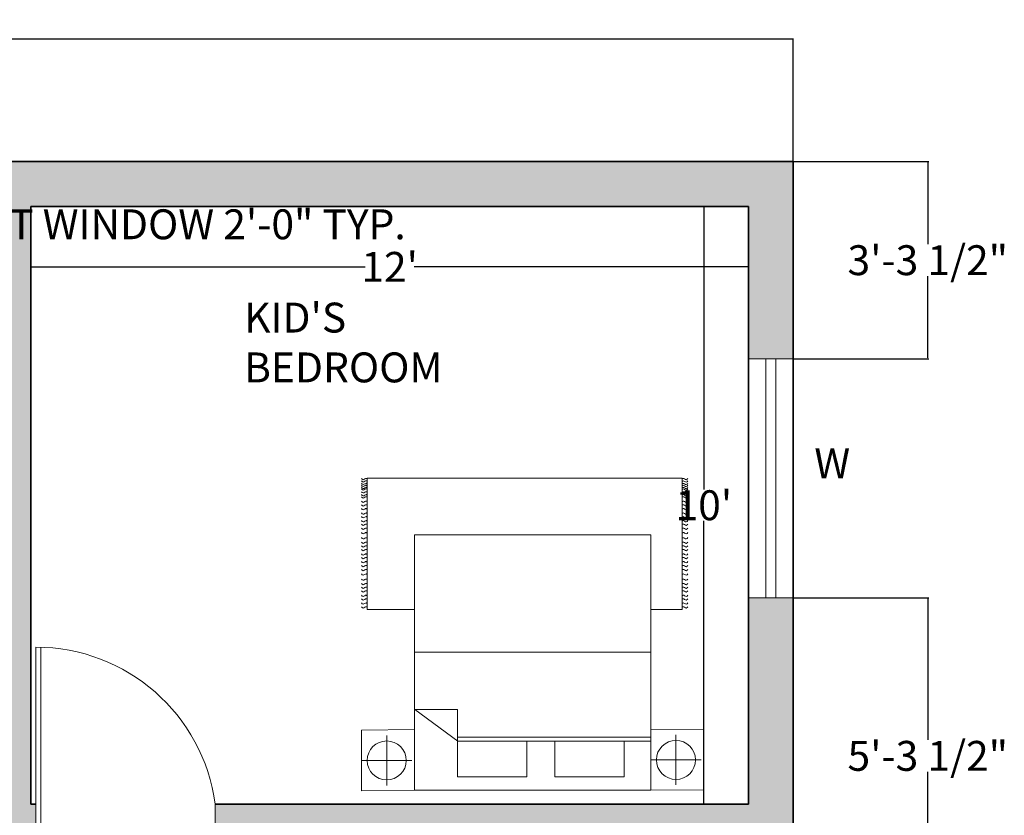
# Model space of a CAD drawing. Units: inches. Extents: x 302 to 1258, y 831 to 1373.
# Tile 6 of 13: x 569 to 767, y 1211 to 1371. Entities that reach past the tile are written whole.
import ezdxf

# ---------------------------------------------------------------- set-up
doc = ezdxf.new("R2010")
doc.units = ezdxf.units.IN
doc.header["$MEASUREMENT"] = 0
for name, color, linetype, lineweight in [('A-ANNO-DIMS', 2, 'Continuous', 18), ('A-ANNO-TEXT', 7, 'Continuous', 18), ('A-AREA-IDEN', 7, 'Continuous', 18), ('A-DOOR', 3, 'Continuous', 18), ('A-FURN', 8, 'Continuous', 18), ('A-GLAZ', 4, 'Continuous', 18), ('A-WALL', 7, 'Continuous', 35), ('A-WALL-PATT', 251, 'Continuous', 13)]:
    doc.layers.add(name, color=color, linetype=linetype, lineweight=lineweight)
doc.styles.get("Standard").update_dxf_attribs({"font": 'arial.ttf'})
doc.dimstyles.get("Standard").update_dxf_attribs({"dimtxt": 6, "dimasz": 0.18, "dimexe": 0.18, "dimexo": 0.0625, "dimgap": 0.09, "dimtad": 0, "dimtih": 1, "dimtoh": 1, "dimdec": 1, "dimzin": 0, "dimdsep": 46, "dimlunit": 3, "dimtxsty": 'Standard', "dimcen": 0.09, "dimadec": 0, "dimazin": 0, "dimtfac": 1, "dimtdec": 1, "dimtofl": 0, "dimtmove": 0, "dimatfit": 3, "dimfxl": 1, "dimtolj": 1, "dimtzin": 0, "dimarcsym": 0})

# ---------------------------------------------------------------- blocks, each defined once
blk = doc.blocks.new('*D7')
at = {"layer": 'A-ANNO-DIMS', "color": 0, "lineweight": -2, "transparency": 16777216}
for p, q in [((571.67, 1333.26), (571.67, 1320.99)), ((715.67, 1333.26), (715.67, 1320.99)), ((571.85, 1321.17), (638.77, 1321.17)), ((715.49, 1321.17), (648.57, 1321.17))]:
    blk.add_line(p, q, dxfattribs=at)
at = {"layer": 'A-ANNO-DIMS', "color": 0, "transparency": 16777216}
for points in [[(571.85, 1321.2), (571.85, 1321.14), (571.67, 1321.17)], [(715.49, 1321.2), (715.49, 1321.14), (715.67, 1321.17)]]:
    blk.add_solid(points, dxfattribs=at)
at = {"layer": 'Defpoints', "color": 0, "transparency": 16777216}
for p in [(571.67, 1333.32), (715.67, 1333.32), (715.67, 1321.17)]:
    blk.add_point(p, dxfattribs=at)
at = {"layer": 'A-ANNO-DIMS', "color": 0, "transparency": 16777216, "insert": (643.67, 1321.17), "char_height": 6, "attachment_point": 5}
blk.add_mtext("\\A1;12'", dxfattribs=at)
blk = doc.blocks.new('*D8')
at = {"layer": 'A-ANNO-DIMS', "color": 0, "lineweight": -2, "transparency": 16777216}
for p, q in [((715.61, 1333.32), (706.55, 1333.32)), ((706.73, 1333.14), (706.73, 1276.47)), ((706.73, 1213.5), (706.73, 1270.17)), ((715.61, 1213.32), (706.55, 1213.32))]:
    blk.add_line(p, q, dxfattribs=at)
at = {"layer": 'A-ANNO-DIMS', "color": 0, "transparency": 16777216}
for points in [[(706.7, 1333.14), (706.76, 1333.14), (706.73, 1333.32)], [(706.7, 1213.5), (706.76, 1213.5), (706.73, 1213.32)]]:
    blk.add_solid(points, dxfattribs=at)
at = {"layer": 'Defpoints', "color": 0, "transparency": 16777216}
for p in [(715.67, 1333.32), (706.73, 1213.32), (715.67, 1213.32)]:
    blk.add_point(p, dxfattribs=at)
at = {"layer": 'A-ANNO-DIMS', "color": 0, "transparency": 16777216, "insert": (706.73, 1273.32), "char_height": 6, "attachment_point": 5}
blk.add_mtext("\\A1;10'", dxfattribs=at)
blk = doc.blocks.new('*D31')
at = {"layer": 'A-ANNO-DIMS', "color": 0, "lineweight": -2, "transparency": 16777216}
for p, q in [((367.67, 1342.38), (367.67, 1367.04)), ((367.85, 1366.86), (532.23, 1366.86)), ((724.49, 1366.86), (560.11, 1366.86)), ((724.67, 1342.38), (724.67, 1367.04))]:
    blk.add_line(p, q, dxfattribs=at)
at = {"layer": 'A-ANNO-DIMS', "color": 0, "transparency": 16777216}
for points in [[(367.85, 1366.89), (367.85, 1366.83), (367.67, 1366.86)], [(724.49, 1366.89), (724.49, 1366.83), (724.67, 1366.86)]]:
    blk.add_solid(points, dxfattribs=at)
at = {"layer": 'Defpoints', "color": 0, "transparency": 16777216}
for p in [(724.67, 1366.86), (367.67, 1342.32), (724.67, 1342.32)]:
    blk.add_point(p, dxfattribs=at)
at = {"layer": 'A-ANNO-DIMS', "color": 0, "transparency": 16777216, "insert": (546.17, 1366.86), "char_height": 6, "attachment_point": 5}
blk.add_mtext('\\A1;29\'-9.0"', dxfattribs=at)
blk = doc.blocks.new('BED-DOUBLE-WITH-NIGHTSTANDS')
for p, q in [((1.12, 36.41), (1.12, 62.78)), ((1.12, 62.78), (64.36, 62.78)), ((64.36, 62.78), (64.36, 36.41)), ((10.66, 36.41), (1.12, 36.41)), ((64.36, 36.41), (58.06, 36.41)), ((10.66, 27.82), (58.08, 27.82)), ((19.27, 16.32), (10.71, 16.32)), ((19.32, 9.97), (10.71, 16.32)), ((19.27, 9.97), (19.27, 16.32)), ((5.06, 1.07), (5.06, 11.12)), ((19.27, 10.78), (58.08, 10.78)), ((19.32, 9.97), (58.08, 9.97)), ((63.11, 1.17), (63.11, 11.22)), ((0.03, 6.09), (10.09, 6.09)), ((58.08, 6.2), (68.14, 6.2))]:
    blk.add_line(p, q)
for points in [[(10.66, 0.1), (10.66, 51.42), (58.08, 51.42), (58.08, 0.1)], [(10.66, 12.29), (0.03, 12.19), (0.03, 0), (10.66, 0.1)], [(68.71, 12.39), (58.08, 12.29), (58.08, 0.1), (68.71, 0.2)], [(19.27, 2.8), (19.27, 9.97), (33.16, 9.97), (33.16, 2.8)], [(38.83, 2.8), (38.83, 9.97), (52.73, 9.97), (52.73, 2.8)]]:
    blk.add_lwpolyline(points, close=True)
for centre in [(5.06, 6.09), (63.11, 6.2)]:
    blk.add_circle(centre, 3.92)
for points, knots in [([(0, 62.71), (0.1, 62.59), (0.29, 62.35), (0.63, 62.59), (0.91, 62.76), (1.06, 62.66), (1.13, 62.61)], [0, 0, 0, 0, 0.400747, 0.791423, 1.067667, 1.29709, 1.29709, 1.29709, 1.29709]), ([(0, 62.24), (0.1, 62.12), (0.29, 61.88), (0.63, 62.12), (0.91, 62.29), (1.06, 62.18), (1.13, 62.13)], [0, 0, 0, 0, 0.400747, 0.791423, 1.067667, 1.29709, 1.29709, 1.29709, 1.29709]), ([(0, 61.75), (0.1, 61.63), (0.29, 61.39), (0.63, 61.63), (0.91, 61.8), (1.06, 61.7), (1.13, 61.65)], [0, 0, 0, 0, 0.400747, 0.791423, 1.067667, 1.29709, 1.29709, 1.29709, 1.29709]), ([(0, 61.35), (0.1, 61.23), (0.29, 60.99), (0.63, 61.23), (0.91, 61.41), (1.06, 61.3), (1.13, 61.25)], [0, 0, 0, 0, 0.400747, 0.791423, 1.067667, 1.29709, 1.29709, 1.29709, 1.29709]), ([(65.48, 62.71), (65.39, 62.59), (65.19, 62.35), (64.85, 62.59), (64.57, 62.76), (64.42, 62.66), (64.36, 62.61)], [0, 0, 0, 0, 0.400747, 0.791423, 1.067667, 1.29709, 1.29709, 1.29709, 1.29709]), ([(65.48, 62.21), (65.39, 62.09), (65.19, 61.85), (64.85, 62.09), (64.57, 62.26), (64.42, 62.15), (64.36, 62.11)], [0, 0, 0, 0, 0.400747, 0.791423, 1.067667, 1.29709, 1.29709, 1.29709, 1.29709]), ([(65.48, 61.72), (65.39, 61.6), (65.19, 61.36), (64.85, 61.6), (64.57, 61.78), (64.42, 61.67), (64.36, 61.62)], [0, 0, 0, 0, 0.400747, 0.791423, 1.067667, 1.29709, 1.29709, 1.29709, 1.29709]), ([(65.48, 61.33), (65.39, 61.21), (65.19, 60.97), (64.85, 61.21), (64.57, 61.38), (64.42, 61.27), (64.36, 61.22)], [0, 0, 0, 0, 0.400747, 0.791423, 1.067667, 1.29709, 1.29709, 1.29709, 1.29709]), ([(0, 60.94), (0.1, 60.81), (0.29, 60.58), (0.63, 60.81), (0.91, 60.99), (1.05, 60.89), (1.12, 60.84)], [0, 0, 0, 0, 0.400747, 0.791423, 1.067667, 1.283686, 1.283686, 1.283686, 1.283686]), ([(0, 60.63), (0.1, 60.51), (0.29, 60.27), (0.63, 60.51), (0.91, 60.68), (1.05, 60.58), (1.12, 60.53)], [0, 0, 0, 0, 0.400747, 0.791423, 1.067667, 1.283686, 1.283686, 1.283686, 1.283686]), ([(0, 60.05), (0.1, 59.93), (0.29, 59.69), (0.63, 59.93), (0.91, 60.1), (1.05, 60), (1.12, 59.96)], [0, 0, 0, 0, 0.400747, 0.791423, 1.067667, 1.283686, 1.283686, 1.283686, 1.283686]), ([(0, 59.46), (0.1, 59.34), (0.29, 59.09), (0.63, 59.34), (0.91, 59.51), (1.05, 59.41), (1.12, 59.36)], [0, 0, 0, 0, 0.402903, 0.794912, 1.071156, 1.287177, 1.287177, 1.287177, 1.287177]), ([(65.48, 60.91), (65.39, 60.79), (65.19, 60.55), (64.85, 60.79), (64.57, 60.96), (64.42, 60.85), (64.36, 60.81)], [0, 0, 0, 0, 0.400747, 0.791423, 1.067667, 1.29709, 1.29709, 1.29709, 1.29709]), ([(65.48, 60.6), (65.39, 60.48), (65.19, 60.24), (64.85, 60.48), (64.57, 60.65), (64.42, 60.54), (64.36, 60.5)], [0, 0, 0, 0, 0.400747, 0.791423, 1.067667, 1.29709, 1.29709, 1.29709, 1.29709]), ([(65.48, 60.03), (65.39, 59.9), (65.19, 59.67), (64.85, 59.9), (64.57, 60.08), (64.42, 59.97), (64.36, 59.92)], [0, 0, 0, 0, 0.400747, 0.791423, 1.067667, 1.29709, 1.29709, 1.29709, 1.29709]), ([(65.48, 59.46), (65.39, 59.33), (65.2, 59.08), (64.85, 59.34), (64.57, 59.51), (64.42, 59.4), (64.36, 59.36)], [0, 0, 0, 0, 0.407265, 0.802015, 1.07826, 1.307683, 1.307683, 1.307683, 1.307683]), ([(0, 59.03), (0.1, 58.91), (0.29, 58.67), (0.63, 58.91), (0.91, 59.08), (1.05, 58.98), (1.12, 58.93)], [0, 0, 0, 0, 0.400747, 0.791423, 1.067667, 1.283686, 1.283686, 1.283686, 1.283686]), ([(0, 58.15), (0.1, 58.03), (0.29, 57.79), (0.63, 58.03), (0.91, 58.2), (1.05, 58.1), (1.12, 58.05)], [0, 0, 0, 0, 0.400747, 0.791423, 1.067667, 1.283686, 1.283686, 1.283686, 1.283686]), ([(0, 57.42), (0.1, 57.3), (0.29, 57.06), (0.63, 57.3), (0.91, 57.47), (1.06, 57.36), (1.13, 57.32)], [0, 0, 0, 0, 0.400747, 0.791423, 1.067667, 1.29709, 1.29709, 1.29709, 1.29709]), ([(65.48, 59.03), (65.39, 58.91), (65.19, 58.67), (64.85, 58.91), (64.57, 59.08), (64.42, 58.97), (64.36, 58.93)], [0, 0, 0, 0, 0.400747, 0.791423, 1.067667, 1.29709, 1.29709, 1.29709, 1.29709]), ([(65.48, 58.15), (65.39, 58.03), (65.19, 57.79), (64.85, 58.03), (64.57, 58.2), (64.42, 58.09), (64.36, 58.04)], [0, 0, 0, 0, 0.400747, 0.791423, 1.067667, 1.29709, 1.29709, 1.29709, 1.29709]), ([(65.48, 57.42), (65.39, 57.3), (65.19, 57.06), (64.85, 57.3), (64.57, 57.47), (64.42, 57.36), (64.36, 57.32)], [0, 0, 0, 0, 0.400747, 0.791423, 1.067667, 1.29709, 1.29709, 1.29709, 1.29709]), ([(0, 56.67), (0.1, 56.55), (0.29, 56.31), (0.63, 56.55), (0.91, 56.72), (1.06, 56.61), (1.13, 56.56)], [0, 0, 0, 0, 0.400747, 0.791423, 1.067667, 1.29709, 1.29709, 1.29709, 1.29709]), ([(0, 55.78), (0.1, 55.66), (0.29, 55.42), (0.63, 55.66), (0.91, 55.84), (1.06, 55.73), (1.13, 55.68)], [0, 0, 0, 0, 0.400747, 0.791423, 1.067667, 1.29709, 1.29709, 1.29709, 1.29709]), ([(65.48, 56.67), (65.39, 56.55), (65.19, 56.31), (64.85, 56.55), (64.57, 56.72), (64.42, 56.61), (64.36, 56.56)], [0, 0, 0, 0, 0.400747, 0.791423, 1.067667, 1.29709, 1.29709, 1.29709, 1.29709]), ([(65.48, 55.78), (65.39, 55.66), (65.19, 55.42), (64.85, 55.66), (64.57, 55.84), (64.42, 55.73), (64.36, 55.68)], [0, 0, 0, 0, 0.400747, 0.791423, 1.067667, 1.29709, 1.29709, 1.29709, 1.29709]), ([(0, 55.06), (0.1, 54.94), (0.29, 54.7), (0.63, 54.94), (0.91, 55.11), (1.06, 55), (1.13, 54.95)], [0, 0, 0, 0, 0.400747, 0.791423, 1.067667, 1.29709, 1.29709, 1.29709, 1.29709]), ([(0, 54.24), (0.1, 54.12), (0.29, 53.88), (0.63, 54.12), (0.91, 54.29), (1.06, 54.19), (1.13, 54.14)], [0, 0, 0, 0, 0.400747, 0.791423, 1.067667, 1.29709, 1.29709, 1.29709, 1.29709]), ([(0, 53.55), (0.1, 53.43), (0.29, 53.19), (0.63, 53.43), (0.91, 53.6), (1.06, 53.5), (1.13, 53.45)], [0, 0, 0, 0, 0.400747, 0.791423, 1.067667, 1.29709, 1.29709, 1.29709, 1.29709]), ([(65.48, 55.06), (65.39, 54.94), (65.19, 54.7), (64.85, 54.94), (64.57, 55.11), (64.42, 55), (64.36, 54.95)], [0, 0, 0, 0, 0.400747, 0.791423, 1.067667, 1.29709, 1.29709, 1.29709, 1.29709]), ([(65.48, 54.24), (65.39, 54.12), (65.19, 53.88), (64.85, 54.12), (64.57, 54.29), (64.42, 54.19), (64.36, 54.14)], [0, 0, 0, 0, 0.400747, 0.791423, 1.067667, 1.29709, 1.29709, 1.29709, 1.29709]), ([(65.48, 53.55), (65.39, 53.43), (65.19, 53.19), (64.85, 53.43), (64.57, 53.6), (64.42, 53.5), (64.36, 53.45)], [0, 0, 0, 0, 0.400747, 0.791423, 1.067667, 1.29709, 1.29709, 1.29709, 1.29709]), ([(0, 52.73), (0.1, 52.61), (0.29, 52.37), (0.63, 52.61), (0.91, 52.79), (1.06, 52.68), (1.13, 52.63)], [0, 0, 0, 0, 0.400747, 0.791423, 1.067667, 1.29709, 1.29709, 1.29709, 1.29709]), ([(0, 51.85), (0.1, 51.73), (0.29, 51.49), (0.63, 51.73), (0.91, 51.9), (1.06, 51.8), (1.13, 51.75)], [0, 0, 0, 0, 0.400747, 0.791423, 1.067667, 1.29709, 1.29709, 1.29709, 1.29709]), ([(65.48, 52.73), (65.39, 52.61), (65.19, 52.37), (64.85, 52.61), (64.57, 52.79), (64.42, 52.68), (64.36, 52.63)], [0, 0, 0, 0, 0.400747, 0.791423, 1.067667, 1.29709, 1.29709, 1.29709, 1.29709]), ([(65.48, 51.85), (65.39, 51.73), (65.19, 51.49), (64.85, 51.73), (64.57, 51.9), (64.42, 51.8), (64.36, 51.75)], [0, 0, 0, 0, 0.400747, 0.791423, 1.067667, 1.29709, 1.29709, 1.29709, 1.29709]), ([(0, 50.82), (0.1, 50.69), (0.29, 50.46), (0.63, 50.69), (0.91, 50.87), (1.06, 50.76), (1.13, 50.71)], [0, 0, 0, 0, 0.400747, 0.791423, 1.067667, 1.29709, 1.29709, 1.29709, 1.29709]), ([(0, 49.93), (0.1, 49.81), (0.29, 49.57), (0.63, 49.81), (0.91, 49.99), (1.06, 49.88), (1.13, 49.83)], [0, 0, 0, 0, 0.400747, 0.791423, 1.067667, 1.29709, 1.29709, 1.29709, 1.29709]), ([(65.48, 50.82), (65.39, 50.69), (65.19, 50.46), (64.85, 50.69), (64.57, 50.87), (64.42, 50.76), (64.36, 50.71)], [0, 0, 0, 0, 0.400747, 0.791423, 1.067667, 1.29709, 1.29709, 1.29709, 1.29709]), ([(65.48, 49.93), (65.39, 49.81), (65.19, 49.57), (64.85, 49.81), (64.57, 49.99), (64.42, 49.88), (64.36, 49.83)], [0, 0, 0, 0, 0.400747, 0.791423, 1.067667, 1.29709, 1.29709, 1.29709, 1.29709]), ([(0, 49.21), (0.1, 49.08), (0.29, 48.84), (0.63, 49.08), (0.91, 49.26), (1.06, 49.15), (1.13, 49.1)], [0, 0, 0, 0, 0.400747, 0.791423, 1.067667, 1.29709, 1.29709, 1.29709, 1.29709]), ([(0, 48.45), (0.1, 48.33), (0.29, 48.09), (0.63, 48.33), (0.91, 48.51), (1.06, 48.4), (1.13, 48.35)], [0, 0, 0, 0, 0.400747, 0.791423, 1.067667, 1.29709, 1.29709, 1.29709, 1.29709]), ([(0, 47.57), (0.1, 47.45), (0.29, 47.21), (0.63, 47.45), (0.91, 47.62), (1.06, 47.52), (1.13, 47.47)], [0, 0, 0, 0, 0.400747, 0.791423, 1.067667, 1.29709, 1.29709, 1.29709, 1.29709]), ([(65.48, 49.21), (65.39, 49.08), (65.19, 48.84), (64.85, 49.08), (64.57, 49.26), (64.42, 49.15), (64.36, 49.1)], [0, 0, 0, 0, 0.400747, 0.791423, 1.067667, 1.29709, 1.29709, 1.29709, 1.29709]), ([(65.48, 48.45), (65.39, 48.33), (65.19, 48.09), (64.85, 48.33), (64.57, 48.51), (64.42, 48.4), (64.36, 48.35)], [0, 0, 0, 0, 0.400747, 0.791423, 1.067667, 1.29709, 1.29709, 1.29709, 1.29709]), ([(65.48, 47.57), (65.39, 47.45), (65.19, 47.21), (64.85, 47.45), (64.57, 47.62), (64.42, 47.52), (64.36, 47.47)], [0, 0, 0, 0, 0.400747, 0.791423, 1.067667, 1.29709, 1.29709, 1.29709, 1.29709]), ([(0, 46.84), (0.1, 46.72), (0.29, 46.48), (0.63, 46.72), (0.91, 46.89), (1.06, 46.79), (1.13, 46.74)], [0, 0, 0, 0, 0.400747, 0.791423, 1.067667, 1.29709, 1.29709, 1.29709, 1.29709]), ([(0, 46.03), (0.1, 45.91), (0.29, 45.67), (0.63, 45.91), (0.91, 46.08), (1.06, 45.97), (1.13, 45.92)], [0, 0, 0, 0, 0.400747, 0.791423, 1.067667, 1.29709, 1.29709, 1.29709, 1.29709]), ([(65.48, 46.84), (65.39, 46.72), (65.19, 46.48), (64.85, 46.72), (64.57, 46.89), (64.42, 46.79), (64.36, 46.74)], [0, 0, 0, 0, 0.400747, 0.791423, 1.067667, 1.29709, 1.29709, 1.29709, 1.29709]), ([(65.48, 46.03), (65.39, 45.91), (65.19, 45.67), (64.85, 45.91), (64.57, 46.08), (64.42, 45.97), (64.36, 45.92)], [0, 0, 0, 0, 0.400747, 0.791423, 1.067667, 1.29709, 1.29709, 1.29709, 1.29709]), ([(0, 45.25), (0.1, 45.13), (0.29, 44.89), (0.63, 45.13), (0.91, 45.3), (1.06, 45.2), (1.13, 45.15)], [0, 0, 0, 0, 0.400747, 0.791423, 1.067667, 1.29709, 1.29709, 1.29709, 1.29709]), ([(0, 44.43), (0.1, 44.31), (0.29, 44.07), (0.63, 44.31), (0.91, 44.49), (1.06, 44.38), (1.13, 44.33)], [0, 0, 0, 0, 0.400747, 0.791423, 1.067667, 1.29709, 1.29709, 1.29709, 1.29709]), ([(0, 43.55), (0.1, 43.43), (0.29, 43.19), (0.63, 43.43), (0.91, 43.6), (1.06, 43.5), (1.13, 43.45)], [0, 0, 0, 0, 0.400747, 0.791423, 1.067667, 1.29709, 1.29709, 1.29709, 1.29709]), ([(65.48, 45.25), (65.39, 45.13), (65.19, 44.89), (64.85, 45.13), (64.57, 45.3), (64.42, 45.2), (64.36, 45.15)], [0, 0, 0, 0, 0.400747, 0.791423, 1.067667, 1.29709, 1.29709, 1.29709, 1.29709]), ([(65.48, 44.43), (65.39, 44.31), (65.19, 44.07), (64.85, 44.31), (64.57, 44.49), (64.42, 44.38), (64.36, 44.33)], [0, 0, 0, 0, 0.400747, 0.791423, 1.067667, 1.29709, 1.29709, 1.29709, 1.29709]), ([(65.48, 43.55), (65.39, 43.43), (65.19, 43.19), (64.85, 43.43), (64.57, 43.6), (64.42, 43.5), (64.36, 43.45)], [0, 0, 0, 0, 0.400747, 0.791423, 1.067667, 1.29709, 1.29709, 1.29709, 1.29709]), ([(0, 42.52), (0.1, 42.39), (0.29, 42.15), (0.63, 42.39), (0.91, 42.57), (1.06, 42.46), (1.13, 42.41)], [0, 0, 0, 0, 0.400747, 0.791423, 1.067667, 1.29709, 1.29709, 1.29709, 1.29709]), ([(0, 41.63), (0.1, 41.51), (0.29, 41.27), (0.63, 41.51), (0.91, 41.68), (1.06, 41.58), (1.13, 41.53)], [0, 0, 0, 0, 0.400747, 0.791423, 1.067667, 1.29709, 1.29709, 1.29709, 1.29709]), ([(65.48, 42.52), (65.39, 42.39), (65.19, 42.15), (64.85, 42.39), (64.57, 42.57), (64.42, 42.46), (64.36, 42.41)], [0, 0, 0, 0, 0.400747, 0.791423, 1.067667, 1.29709, 1.29709, 1.29709, 1.29709]), ([(65.48, 41.63), (65.39, 41.51), (65.19, 41.27), (64.85, 41.51), (64.57, 41.68), (64.42, 41.58), (64.36, 41.53)], [0, 0, 0, 0, 0.400747, 0.791423, 1.067667, 1.29709, 1.29709, 1.29709, 1.29709]), ([(0, 40.9), (0.1, 40.78), (0.29, 40.54), (0.63, 40.78), (0.91, 40.96), (1.06, 40.85), (1.13, 40.8)], [0, 0, 0, 0, 0.400747, 0.791423, 1.067667, 1.29709, 1.29709, 1.29709, 1.29709]), ([(0, 40.15), (0.1, 40.03), (0.29, 39.79), (0.63, 40.03), (0.91, 40.2), (1.06, 40.1), (1.13, 40.05)], [0, 0, 0, 0, 0.400747, 0.791423, 1.067667, 1.29709, 1.29709, 1.29709, 1.29709]), ([(65.48, 40.9), (65.39, 40.78), (65.19, 40.54), (64.85, 40.78), (64.57, 40.96), (64.42, 40.85), (64.36, 40.8)], [0, 0, 0, 0, 0.400747, 0.791423, 1.067667, 1.29709, 1.29709, 1.29709, 1.29709]), ([(65.48, 40.15), (65.39, 40.03), (65.19, 39.79), (64.85, 40.03), (64.57, 40.2), (64.42, 40.1), (64.36, 40.05)], [0, 0, 0, 0, 0.400747, 0.791423, 1.067667, 1.29709, 1.29709, 1.29709, 1.29709]), ([(0, 39.27), (0.1, 39.15), (0.29, 38.91), (0.63, 39.15), (0.91, 39.32), (1.06, 39.22), (1.13, 39.17)], [0, 0, 0, 0, 0.400747, 0.791423, 1.067667, 1.29709, 1.29709, 1.29709, 1.29709]), ([(0, 38.54), (0.1, 38.42), (0.29, 38.18), (0.63, 38.42), (0.91, 38.59), (1.06, 38.49), (1.13, 38.44)], [0, 0, 0, 0, 0.400747, 0.791423, 1.067667, 1.29709, 1.29709, 1.29709, 1.29709]), ([(0, 37.73), (0.1, 37.61), (0.29, 37.37), (0.63, 37.61), (0.91, 37.78), (1.06, 37.67), (1.13, 37.62)], [0, 0, 0, 0, 0.400747, 0.791423, 1.067667, 1.29709, 1.29709, 1.29709, 1.29709]), ([(65.48, 39.27), (65.39, 39.15), (65.19, 38.91), (64.85, 39.15), (64.57, 39.32), (64.42, 39.22), (64.36, 39.17)], [0, 0, 0, 0, 0.400747, 0.791423, 1.067667, 1.29709, 1.29709, 1.29709, 1.29709]), ([(65.48, 38.54), (65.39, 38.42), (65.19, 38.18), (64.85, 38.42), (64.57, 38.59), (64.42, 38.49), (64.36, 38.44)], [0, 0, 0, 0, 0.400747, 0.791423, 1.067667, 1.29709, 1.29709, 1.29709, 1.29709]), ([(65.48, 37.73), (65.39, 37.61), (65.19, 37.37), (64.85, 37.61), (64.57, 37.78), (64.42, 37.67), (64.36, 37.62)], [0, 0, 0, 0, 0.400747, 0.791423, 1.067667, 1.29709, 1.29709, 1.29709, 1.29709]), ([(0, 36.95), (0.1, 36.83), (0.29, 36.59), (0.63, 36.83), (0.91, 37), (1.06, 36.89), (1.13, 36.85)], [0, 0, 0, 0, 0.400747, 0.791423, 1.067667, 1.29709, 1.29709, 1.29709, 1.29709]), ([(65.48, 36.95), (65.39, 36.83), (65.19, 36.59), (64.85, 36.83), (64.57, 37), (64.42, 36.89), (64.36, 36.85)], [0, 0, 0, 0, 0.400747, 0.791423, 1.067667, 1.29709, 1.29709, 1.29709, 1.29709])]:
    blk.add_open_spline(points, degree=3, knots=knots)
blk = doc.blocks.new('WINDOW-48IN')
for p, q in [((0, 0), (0, 9)), ((0, 9), (48, 9)), ((48, 9), (48, 0)), ((0, 5.5), (48, 5.5)), ((48, 3.5), (0, 3.5)), ((48, 0), (0, 0))]:
    blk.add_line(p, q)
blk = doc.blocks.new('DOOR-36IN-BEDROOM')
for p, q in [((35, 36), (35, 0)), ((36, 0), (36, 36)), ((36, 36), (36, 0)), ((0, 0), (0, 4.5)), ((36, 0), (0, 0)), ((37, 0), (36, 0))]:
    blk.add_line(p, q)
blk.add_arc((36, -0.32), 36.32, 90, 172.3719)
blk = doc.blocks.new('*D53')
at = {"layer": 'A-ANNO-DIMS', "color": 0, "lineweight": -2, "transparency": 16777216}
for p, q in [((524.78, 1333.26), (524.78, 1329.54)), ((548.78, 1333.26), (548.78, 1329.54)), ((524.96, 1329.72), (548.6, 1329.72)), ((548.78, 1329.72), (548.96, 1329.72))]:
    blk.add_line(p, q, dxfattribs=at)
at = {"layer": 'A-ANNO-DIMS', "color": 0, "transparency": 16777216}
for points in [[(524.96, 1329.75), (524.96, 1329.69), (524.78, 1329.72)], [(548.6, 1329.75), (548.6, 1329.69), (548.78, 1329.72)]]:
    blk.add_solid(points, dxfattribs=at)
at = {"layer": 'Defpoints', "color": 0, "transparency": 16777216}
for p in [(524.78, 1333.32), (548.78, 1333.32), (548.78, 1329.72)]:
    blk.add_point(p, dxfattribs=at)
at = {"layer": 'A-ANNO-DIMS', "color": 0, "transparency": 16777216, "insert": (599.38, 1329.72), "char_height": 6, "attachment_point": 5}
blk.add_mtext('\\A1;VENT WINDOW 2\'-0" TYP.', dxfattribs=at)
blk = doc.blocks.new('*D55')
at = {"layer": 'A-ANNO-DIMS', "color": 0, "lineweight": -2, "transparency": 16777216}
for p, q in [((459.67, 1208.76), (459.67, 1203.09)), ((496.67, 1208.76), (496.67, 1203.09)), ((459.85, 1203.27), (496.49, 1203.27)), ((496.67, 1203.27), (496.85, 1203.27))]:
    blk.add_line(p, q, dxfattribs=at)
at = {"layer": 'A-ANNO-DIMS', "color": 0, "transparency": 16777216}
for points in [[(459.85, 1203.3), (459.85, 1203.24), (459.67, 1203.27)], [(496.49, 1203.3), (496.49, 1203.24), (496.67, 1203.27)]]:
    blk.add_solid(points, dxfattribs=at)
at = {"layer": 'Defpoints', "color": 0, "transparency": 16777216}
for p in [(459.67, 1208.82), (496.67, 1208.82), (496.67, 1203.27)]:
    blk.add_point(p, dxfattribs=at)
at = {"layer": 'A-ANNO-DIMS', "color": 0, "transparency": 16777216, "insert": (551.65, 1203.27), "char_height": 6, "attachment_point": 5}
blk.add_mtext('\\A1;BEDROOM DOOR 3\'-1" TYP.', dxfattribs=at)
blk = doc.blocks.new('*D75')
at = {"layer": 'A-ANNO-DIMS', "color": 0, "lineweight": -2, "transparency": 16777216}
for p, q in [((724.73, 1342.32), (751.85, 1342.32)), ((751.67, 1342.14), (751.67, 1325.71)), ((751.67, 1302.89), (751.67, 1319.32)), ((724.73, 1302.71), (751.85, 1302.71))]:
    blk.add_line(p, q, dxfattribs=at)
at = {"layer": 'A-ANNO-DIMS', "color": 0, "transparency": 16777216}
for points in [[(751.64, 1342.14), (751.7, 1342.14), (751.67, 1342.32)], [(751.64, 1302.89), (751.7, 1302.89), (751.67, 1302.71)]]:
    blk.add_solid(points, dxfattribs=at)
at = {"layer": 'Defpoints', "color": 0, "transparency": 16777216}
for p in [(724.67, 1342.32), (724.67, 1302.71), (751.67, 1302.71)]:
    blk.add_point(p, dxfattribs=at)
at = {"layer": 'A-ANNO-DIMS', "color": 0, "transparency": 16777216, "insert": (751.67, 1322.51), "char_height": 6, "attachment_point": 5}
blk.add_mtext('\\A1;3\'-3 1/2"', dxfattribs=at)
blk = doc.blocks.new('*D76')
at = {"layer": 'A-ANNO-DIMS', "color": 0, "lineweight": -2, "transparency": 16777216}
for p, q in [((724.73, 1254.71), (751.85, 1254.71)), ((751.67, 1254.53), (751.67, 1226.2)), ((751.67, 1191.48), (751.67, 1219.81)), ((724.73, 1191.3), (751.85, 1191.3))]:
    blk.add_line(p, q, dxfattribs=at)
at = {"layer": 'A-ANNO-DIMS', "color": 0, "transparency": 16777216}
for points in [[(751.64, 1254.53), (751.7, 1254.53), (751.67, 1254.71)], [(751.64, 1191.48), (751.7, 1191.48), (751.67, 1191.3)]]:
    blk.add_solid(points, dxfattribs=at)
at = {"layer": 'Defpoints', "color": 0, "transparency": 16777216}
for p in [(724.67, 1254.71), (724.67, 1191.3), (751.67, 1191.3)]:
    blk.add_point(p, dxfattribs=at)
at = {"layer": 'A-ANNO-DIMS', "color": 0, "transparency": 16777216, "insert": (751.67, 1223), "char_height": 6, "attachment_point": 5}
blk.add_mtext('\\A1;5\'-3 1/2"', dxfattribs=at)

msp = doc.modelspace()

# ---------------------------------------------------------------- hatches: boundary and pattern name
at = {"layer": 'A-WALL-PATT'}
h = msp.add_hatch(color=256, dxfattribs=at)
h.dxf.hatch_style = 1
h.paths.add_polyline_path([(524.78, 1342.32), (455.57, 1342.32), (455.57, 1333.32), (496.67, 1333.32), (496.67, 1330.32), (501.17, 1330.32), (501.17, 1333.32), (524.78, 1333.32)])
h.paths.add_polyline_path([(724.67, 1342.32), (548.78, 1342.32), (548.78, 1333.32), (567.17, 1333.32), (567.17, 1213.32), (501.17, 1213.32), (501.17, 1306.32), (496.67, 1306.32), (496.67, 1213.32), (495.67, 1213.32), (495.67, 1208.82), (496.67, 1208.82), (572.67, 1208.82), (572.67, 1213.32), (571.67, 1213.32), (571.67, 1333.32), (715.67, 1333.32), (715.67, 1302.71), (724.67, 1302.71)])
h.paths.add_polyline_path([(376.67, 1333.32), (407.57, 1333.32), (407.57, 1342.32), (367.67, 1342.32), (367.67, 1300.76), (376.67, 1300.76)])
h.paths.add_polyline_path([(459.67, 1213.32), (376.67, 1213.32), (376.67, 1252.76), (367.67, 1252.76), (367.67, 1164.55), (376.67, 1164.55), (376.67, 1208.82), (454.67, 1208.82), (454.67, 1082.82), (459.17, 1082.82), (459.17, 1208.82), (459.67, 1208.82)])
h.paths.add_polyline_path([(376.67, 1116.55), (367.67, 1116.55), (367.67, 1024.44), (376.67, 1024.44)])
h.paths.add_polyline_path([(724.67, 1254.71), (715.67, 1254.71), (715.67, 1213.32), (608.67, 1213.32), (608.67, 1208.82), (615.17, 1208.82), (615.17, 1205.82), (619.67, 1205.82), (619.67, 1208.82), (715.67, 1208.82), (715.67, 1191.3), (724.67, 1191.3)])
h.paths.add_polyline_path([(724.67, 1167.3), (715.67, 1167.3), (715.67, 1136.82), (619.67, 1136.82), (619.67, 1181.82), (615.17, 1181.82), (615.17, 1136.82), (591.17, 1136.82), (591.17, 1129.32), (595.67, 1129.32), (595.67, 1132.32), (715.67, 1132.32), (715.67, 1097.42), (724.67, 1097.42)])
h.paths.add_polyline_path([(724.67, 1049.42), (715.67, 1049.42), (715.67, 1012.32), (595.67, 1012.32), (595.67, 1093.32), (591.17, 1093.32), (591.17, 1007.82), (715.67, 1007.82), (715.67, 875.82), (709.67, 875.82), (709.67, 866.82), (715.67, 866.82), (724.67, 866.82)])
h.paths.add_polyline_path([(673.67, 875.82), (623.88, 875.82), (623.88, 866.82), (673.67, 866.82)], flags=17)
h.paths.add_polyline_path([(575.88, 875.82), (477.17, 875.82), (477.17, 971.82), (472.67, 971.82), (472.67, 875.82), (376.67, 875.82), (376.67, 896.2), (367.67, 896.2), (367.67, 866.82), (575.88, 866.82)])
h.paths.add_polyline_path([(376.67, 976.44), (367.67, 976.44), (367.67, 944.2), (376.67, 944.2)])

# ---------------------------------------------------------------- linework, layer by layer
at = {"layer": 'A-WALL'}
for p, q in [((367.67, 1342.32), (724.67, 1342.32)), ((724.67, 1342.32), (724.67, 866.82)), ((571.67, 1333.32), (571.67, 1213.32)), ((571.67, 1333.32), (715.67, 1333.32)), ((715.67, 1333.32), (715.67, 1213.32)), ((571.67, 1213.32), (572.67, 1213.32)), ((608.67, 1213.32), (715.67, 1213.32))]:
    msp.add_line(p, q, dxfattribs=at)

# ---------------------------------------------------------------- block references
at = {"layer": 'A-DOOR', "extrusion": (0, 0, -1), "zscale": -1}
msp.add_blockref('DOOR-36IN-BEDROOM', (-608.67, 1208.82), dxfattribs=at)
at = {"layer": 'A-FURN'}
msp.add_blockref('BED-DOUBLE-WITH-NIGHTSTANDS', (638.02, 1215.99), dxfattribs=at)
at = {"layer": 'A-GLAZ', "rotation": 269.9999999999996}
msp.add_blockref('WINDOW-48IN', (715.67, 1302.71), dxfattribs=at)

# ---------------------------------------------------------------- texts
at = {"layer": 'A-ANNO-TEXT', "insert": (728.9, 1284.74), "char_height": 6, "attachment_point": 1}
msp.add_mtext_dynamic_manual_height_columns('W', width=16.4894, gutter_width=30, heights=[0], dxfattribs=at)
at = {"layer": 'A-AREA-IDEN', "insert": (614.47, 1313.99), "char_height": 6, "attachment_point": 1}
msp.add_mtext_dynamic_manual_height_columns("KID'S\\PBEDROOM", width=58.0496, gutter_width=30, heights=[0], dxfattribs=at)

# ---------------------------------------------------------------- dimensions: what is measured, and where the dimension line sits
at = {"layer": 'A-ANNO-DIMS'}
for base, p1, p2, picture, middle in [((724.67, 1366.86), (367.67, 1342.32), (724.67, 1342.32), '*D31', (546.17, 1366.86)), ((715.67, 1321.17), (571.67, 1333.32), (715.67, 1333.32), '*D7', (643.67, 1321.17))]:
    dim = msp.add_linear_dim(base=base, p1=p1, p2=p2, dimstyle='Standard', override={"dimclrd": 0, "dimclre": 0, "dimclrt": 0}, dxfattribs=at)
    dim.commit()
    dim.dimension.update_dxf_attribs({"geometry": picture, "text_midpoint": middle})
for base, p1, p2, text, picture, middle in [((548.78, 1329.72), (524.78, 1333.32), (548.78, 1333.32), 'VENT WINDOW <> TYP.', '*D53', (599.38, 1329.72)), ((496.67, 1203.27), (459.67, 1208.82), (496.67, 1208.82), 'BEDROOM DOOR <> TYP.', '*D55', (551.65, 1203.27))]:
    dim = msp.add_linear_dim(base=base, p1=p1, p2=p2, text=text, dimstyle='Standard', override={"dimdec": 1, "dimlfac": 1, "dimrnd": 0, "dimzin": 1, "dimdsep": 46, "dimlunit": 4, "dimfrac": 2}, dxfattribs=at)
    dim.commit()
    dim.dimension.update_dxf_attribs({"geometry": picture, "text_midpoint": middle})
for base, p1, p2, override, picture, middle in [((751.67, 1302.71), (724.67, 1342.32), (724.67, 1302.71), {"dimdec": 1, "dimlfac": 1, "dimrnd": 0, "dimzin": 1, "dimdsep": 46, "dimlunit": 4, "dimfrac": 2}, '*D75', (751.67, 1322.51)), ((706.73, 1213.32), (715.67, 1333.32), (715.67, 1213.32), {"dimclrd": 0, "dimclre": 0, "dimclrt": 0}, '*D8', (706.73, 1273.32)), ((751.67, 1191.3), (724.67, 1254.71), (724.67, 1191.3), {"dimdec": 1, "dimlfac": 1, "dimrnd": 0, "dimzin": 1, "dimdsep": 46, "dimlunit": 4, "dimfrac": 2}, '*D76', (751.67, 1223))]:
    dim = msp.add_linear_dim(base=base, p1=p1, p2=p2, angle=90, dimstyle='Standard', override=override, dxfattribs=at)
    dim.commit()
    dim.dimension.update_dxf_attribs({"geometry": picture, "text_midpoint": middle})

doc.saveas('drawing.dxf')
